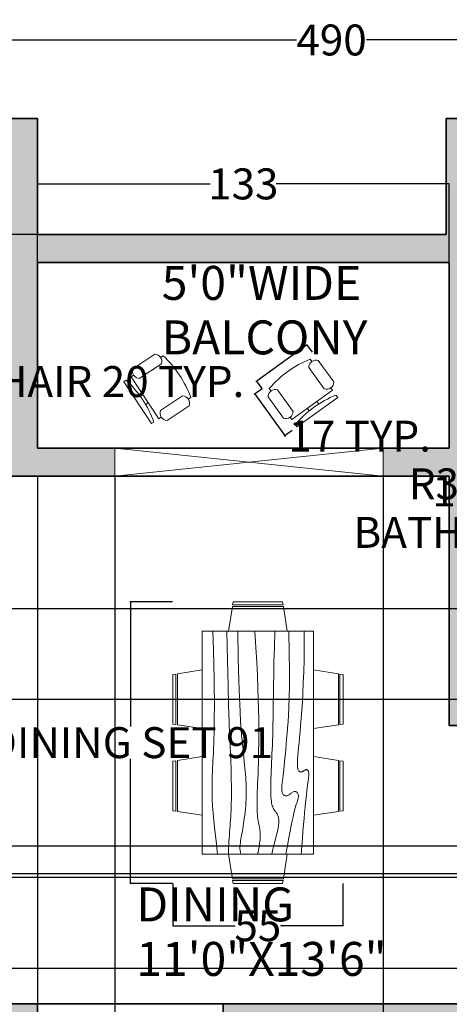
# Model space of a CAD drawing. Units: inches. Extents: x 143 to 746, y -392 to 145.
# Tile 3 of 6: x 334 to 473, y -173 to 145. Entities that reach past the tile are written whole.
import ezdxf

# ---------------------------------------------------------------- set-up
doc = ezdxf.new("R2010")
doc.units = ezdxf.units.IN
doc.header["$MEASUREMENT"] = 0
doc.linetypes.add('ACAD_ISO02W100', pattern=[15, 12, -3])
for name, color, linetype, lineweight in [('A-ANNO-DIMS', 2, 'Continuous', 18), ('A-AREA-IDEN', 7, 'Continuous', 20), ('A-DOOR', 3, 'Continuous', 18), ('A-FURN', 8, 'Continuous', 18), ('A-WALL', 7, 'Continuous', 35), ('A-WALL-OVHD', 7, 'ACAD_ISO02W100', 18)]:
    doc.layers.add(name, color=color, linetype=linetype, lineweight=lineweight)
doc.layers.add('A-WALL-PATT', color=252, linetype='Continuous', lineweight=13, true_color=0x939598)
doc.styles.get("Standard").update_dxf_attribs({"font": 'arial.ttf'})
doc.dimstyles.get("Standard").update_dxf_attribs({"dimtxt": 10, "dimasz": 0.18, "dimexe": 0.18, "dimexo": 0.0625, "dimgap": 0.09, "dimtad": 0, "dimtih": 1, "dimtoh": 1, "dimdec": 0, "dimzin": 0, "dimdsep": 46, "dimlunit": 3, "dimtxsty": 'Standard', "dimcen": 0.09, "dimadec": 0, "dimazin": 0, "dimtfac": 1, "dimtdec": 0, "dimtofl": 0, "dimtmove": 0, "dimatfit": 3, "dimfxl": 1, "dimtolj": 1, "dimtzin": 0, "dimarcsym": 0})

# ---------------------------------------------------------------- blocks, each defined once
blk = doc.blocks.new('Dining Set - 36 x 72 in.')
for p, q in [((-22.2343, 26.00059), (-23.4847, 17.99762)), ((-22.2304, 26), (-5.7608, 26)), ((-22, 27.5), (-22.1562, 26.50042)), ((-5.8416, 26.5), (-22.1534, 26.5)), ((-22, 27.5), (-6, 27.5)), ((-5.8437, 26.49966), (-6, 27.5)), ((-4.5152, 17.99762), (-5.7655, 25.99926)), ((5.7657, 26.00059), (4.5153, 17.99762)), ((5.7696, 26), (22.2392, 26)), ((6, 27.5), (5.8438, 26.50042)), ((22.1584, 26.5), (5.8466, 26.5)), ((6, 27.5), (22, 27.5)), ((22.1563, 26.49966), (22, 27.5)), ((23.4848, 17.99762), (22.2345, 25.99926)), ((36, 18), (-36, 18)), ((-36, 18), (-36, -18)), ((36, -18), (36, 18)), ((-45.5, 8), (-44.5004, 8.15617)), ((-45.5, 8), (-45.5, -8)), ((-44.5, -8.15843), (-44.5, 8.15338)), ((-44.0006, 8.23428), (-35.9976, 9.48474)), ((-44, 8.23041), (-44, -8.23915)), ((44.0006, 8.23428), (35.9976, 9.48474)), ((44, 8.23041), (44, -8.23915)), ((44.5, -8.15843), (44.5, 8.15338)), ((45.5, 8), (44.5005, 8.15617)), ((45.5, 8), (45.5, -8)), ((-44.4997, -8.15631), (-45.5, -8)), ((-35.9976, -9.48476), (-43.9993, -8.2345)), ((35.9976, -9.48476), (43.9993, -8.2345)), ((44.4997, -8.15631), (45.5, -8)), ((-36, -18), (36, -18)), ((-22.2343, -26.0006), (-23.4847, -17.99762)), ((-4.5152, -17.99762), (-5.7655, -25.99928)), ((5.7657, -26.0006), (4.5153, -17.99762)), ((23.4848, -17.99762), (22.2345, -25.99928)), ((-22.2304, -26), (-5.7608, -26)), ((-22, -27.5), (-22.1562, -26.50044)), ((-5.8416, -26.5), (-22.1534, -26.5)), ((-22, -27.5), (-6, -27.5)), ((-5.8437, -26.49967), (-6, -27.5)), ((5.7696, -26), (22.2392, -26)), ((6, -27.5), (5.8438, -26.50044)), ((22.1584, -26.5), (5.8466, -26.5)), ((6, -27.5), (22, -27.5)), ((22.1563, -26.49967), (22, -27.5))]:
    blk.add_line(p, q)
for points in [[(-36, 15), (-31.1772, 14.97754), (-26.8079, 14.91406), (-22.8538, 14.81543), (-19.276, 14.6875), (-16.0362, 14.53613), (-13.0957, 14.36718), (-10.4159, 14.18652), (-7.9583, 14), (-5.6904, 13.81315), (-3.6035, 13.63021), (-1.6954, 13.45508), (0.0365, 13.29166), (1.5945, 13.14388), (2.9811, 13.01562), (4.1988, 12.9108), (5.25, 12.83333), (6.1393, 12.78613), (6.8802, 12.76823), (7.4883, 12.77767), (7.9792, 12.8125), (8.3685, 12.87077), (8.6719, 12.95052), (8.9049, 13.0498), (9.0833, 13.16666), (9.2205, 13.29899), (9.3216, 13.44401), (9.3895, 13.59879), (9.4271, 13.76041), (9.4373, 13.92594), (9.4232, 14.09245), (9.3875, 14.257), (9.3333, 14.41666), (9.2638, 14.56917), (9.1836, 14.71484), (9.0975, 14.85465), (9.0104, 14.98958), (8.9272, 15.1206), (8.8529, 15.2487), (8.7922, 15.37483), (8.75, 15.5), (8.7305, 15.62467), (8.7344, 15.74739), (8.7617, 15.86621), (8.8125, 15.97916), (8.8867, 16.08431), (8.9844, 16.17968), (9.1055, 16.26334), (9.25, 16.33333), (9.4189, 16.38802), (9.6172, 16.42708), (9.8506, 16.45052), (10.125, 16.45833), (10.4463, 16.45052), (10.8203, 16.42708), (11.2529, 16.38802), (11.75, 16.33333), (12.3184, 16.26318), (12.9694, 16.17838), (13.7151, 16.07991), (14.5677, 15.96875), (15.5395, 15.84586), (16.6426, 15.71224), (17.8893, 15.56884), (19.2917, 15.41666), (20.859, 15.25667), (22.5879, 15.08984), (24.4721, 14.91715), (26.5052, 14.73958), (28.6809, 14.5581), (30.9929, 14.3737), (33.4347, 14.18733), (36, 14)], [(-36, 10), (-28.9766, 10.14274), (-23.1725, 10.20442), (-18.4241, 10.19775), (-14.5677, 10.13541), (-11.4399, 10.03011), (-8.877, 9.89453), (-6.7154, 9.74137), (-4.7917, 9.58333), (-2.9698, 9.43082), (-1.2246, 9.28515), (0.4415, 9.14534), (2.026, 9.01041), (3.5266, 8.87939), (4.9408, 8.7513), (6.266, 8.62516), (7.5, 8.5), (8.6411, 8.37549), (9.6914, 8.2539), (10.6538, 8.13818), (11.5312, 8.03125), (12.3267, 7.93603), (13.043, 7.85547), (13.6831, 7.79248), (14.25, 7.75), (14.7471, 7.7303), (15.1797, 7.73307), (15.5537, 7.75732), (15.875, 7.80208), (16.1494, 7.86637), (16.3828, 7.94922), (16.5811, 8.04964), (16.75, 8.16666), (16.8944, 8.29915), (17.0143, 8.44531), (17.1089, 8.60319), (17.1771, 8.77083), (17.218, 8.94629), (17.2305, 9.1276), (17.2137, 9.31282), (17.1667, 9.5), (17.0895, 9.6875), (16.987, 9.875), (16.8649, 10.0625), (16.7292, 10.25), (16.5856, 10.4375), (16.4401, 10.625), (16.2985, 10.8125), (16.1667, 11), (16.05, 11.18733), (15.9518, 11.3737), (15.8752, 11.5581), (15.8229, 11.73958), (15.798, 11.91715), (15.8034, 12.08984), (15.842, 12.25667), (15.9167, 12.41666), (16.0295, 12.56836), (16.1784, 12.70833), (16.3605, 12.83268), (16.5729, 12.9375), (16.8127, 13.01888), (17.0768, 13.07291), (17.3625, 13.0957), (17.6667, 13.08333), (17.9894, 13.03312), (18.3418, 12.94726), (18.7382, 12.82918), (19.1927, 12.68229), (19.7195, 12.51001), (20.3327, 12.31575), (21.0465, 12.10294), (21.875, 11.875), (22.8357, 11.63354), (23.959, 11.37304), (25.2786, 11.08618), (26.8282, 10.76562), (28.6414, 10.40405), (30.752, 9.99414), (33.1936, 9.52856), (36, 9)], [(-36, 5.5), (-30.7157, 5.3348), (-26.069, 5.20963), (-21.9946, 5.11767), (-18.4271, 5.05208), (-15.3009, 5.00602), (-12.5508, 4.97265), (-10.1112, 4.94515), (-7.9167, 4.91666), (-5.909, 4.88167), (-4.0586, 4.83984), (-2.3429, 4.79215), (-0.7396, 4.73958), (0.7739, 4.6831), (2.22, 4.6237), (3.6213, 4.56233), (5, 4.5), (6.373, 4.43782), (7.7344, 4.3776), (9.0723, 4.32129), (10.375, 4.27083), (11.6309, 4.22819), (12.8281, 4.19531), (13.9551, 4.17415), (15, 4.16666), (15.954, 4.17448), (16.819, 4.19791), (17.6001, 4.23698), (18.3021, 4.29166), (18.9299, 4.36198), (19.4883, 4.44791), (19.9823, 4.54948), (20.4167, 4.66666), (20.7969, 4.79899), (21.1302, 4.94401), (21.4245, 5.09879), (21.6875, 5.26041), (21.9271, 5.42594), (22.1511, 5.59245), (22.3672, 5.757), (22.5834, 5.91666), (22.8065, 6.06868), (23.0404, 6.21093), (23.2879, 6.34147), (23.5521, 6.45833), (23.8358, 6.55957), (24.142, 6.64323), (24.4735, 6.70735), (24.8334, 6.75), (25.2235, 6.76969), (25.642, 6.76692), (26.0858, 6.74267), (26.5521, 6.69791), (27.0379, 6.63362), (27.5404, 6.55078), (28.0565, 6.45036), (28.5834, 6.33333), (29.1242, 6.19987), (29.7071, 6.04687), (30.3661, 5.87044), (31.1354, 5.66666), (32.0493, 5.43164), (33.142, 5.16146), (34.4475, 4.85221), (36, 4.5)], [(-36, -1), (-30.7915, -0.6591), (-26.0195, -0.38216), (-21.6519, -0.16284), (-17.6563, 0.00521), (-14.0005, 0.12833), (-10.6523, 0.21289), (-7.5796, 0.26522), (-4.75, 0.29166), (-2.134, 0.29793), (0.2878, 0.28711), (2.5317, 0.26163), (4.6146, 0.22396), (6.5529, 0.17651), (8.3633, 0.12174), (10.0623, 0.06209), (11.6667, 0), (13.1899, -0.06201), (14.6341, -0.1211), (15.9982, -0.17432), (17.2813, -0.21875), (18.4823, -0.25147), (19.6003, -0.26953), (20.6343, -0.27002), (21.5834, -0.25), (22.4481, -0.20768), (23.2357, -0.14584), (23.9549, -0.06836), (24.6146, 0.02083), (25.2235, 0.11784), (25.7904, 0.21875), (26.3241, 0.31966), (26.8334, 0.41666), (27.3265, 0.50618), (27.8099, 0.58593), (28.2894, 0.65397), (28.7709, 0.70833), (29.2601, 0.74707), (29.763, 0.76823), (30.2855, 0.76985), (30.8334, 0.75), (31.4088, 0.70784), (31.9994, 0.64713), (32.589, 0.57275), (33.1615, 0.48958), (33.7008, 0.4025), (34.1908, 0.3164), (34.6153, 0.23616), (34.9584, 0.16666), (35.2099, 0.11165), (35.3848, 0.07031), (35.504, 0.04069), (35.5886, 0.02083), (35.6594, 0.00879), (35.7377, 0.0026), (35.8442, 0.00032), (36, 0)], [(-36, -6.5), (-27.1843, -6.31267), (-20.084, -6.1263), (-14.469, -5.9419), (-10.1094, -5.76042), (-6.7752, -5.58285), (-4.2363, -5.41016), (-2.2629, -5.24333), (-0.625, -5.08334), (0.8708, -4.93099), (2.2715, -4.78646), (3.5872, -4.64974), (4.8281, -4.52084), (6.0046, -4.39974), (7.127, -4.28646), (8.2053, -4.18099), (9.25, -4.08334), (10.2705, -3.99382), (11.2734, -3.91407), (12.2647, -3.84603), (13.25, -3.79167), (14.2354, -3.75293), (15.2266, -3.73177), (16.2295, -3.73015), (17.25, -3.75), (18.2912, -3.79248), (19.3451, -3.85547), (20.4009, -3.93604), (21.4479, -4.03125), (22.4754, -4.13819), (23.4727, -4.25391), (24.4289, -4.37549), (25.3334, -4.5), (26.1785, -4.62492), (26.9694, -4.74935), (27.7145, -4.87281), (28.4219, -4.99479), (29.1, -5.11483), (29.7572, -5.23242), (30.4016, -5.34709), (31.0417, -5.45834), (31.6837, -5.56437), (32.3262, -5.65821), (32.9658, -5.73153), (33.599, -5.77604), (34.2224, -5.78345), (34.8327, -5.74545), (35.4264, -5.65373), (36, -5.5)], [(-36, -10), (-26.4022, -9.81299), (-18.4675, -9.62891), (-11.9839, -9.45069), (-6.7396, -9.28125), (-2.5226, -9.12354), (0.8789, -8.98047), (3.6769, -8.85498), (6.0833, -8.75), (8.2767, -8.66765), (10.3021, -8.60677), (12.1712, -8.56543), (13.8958, -8.54167), (15.4876, -8.53353), (16.9583, -8.53907), (18.3197, -8.55632), (19.5834, -8.58334), (20.7616, -8.61841), (21.8685, -8.66081), (22.9188, -8.71004), (23.9271, -8.76563), (24.9081, -8.82707), (25.8763, -8.89388), (26.8465, -8.96558), (27.8334, -9.04167), (28.8474, -9.12118), (29.8828, -9.20117), (30.93, -9.27824), (31.9792, -9.34896), (33.0205, -9.40991), (34.0443, -9.45768), (35.0407, -9.48885), (36, -9.5)], [(-36, -14.5), (-30.0881, -14.33513), (-25.0332, -14.21224), (-20.7312, -14.12647), (-17.0781, -14.07292), (-13.97, -14.04671), (-11.3027, -14.04297), (-8.9724, -14.05681), (-6.875, -14.08334), (-4.9224, -14.11833), (-3.0905, -14.16016), (-1.3709, -14.20785), (0.2448, -14.26042), (1.7647, -14.3169), (3.1973, -14.3763), (4.5507, -14.43767), (5.8333, -14.5), (7.0554, -14.5621), (8.235, -14.62175), (9.3922, -14.67652), (10.5469, -14.72396), (11.7192, -14.76164), (12.929, -14.78711), (14.1965, -14.79794), (15.5417, -14.79167), (16.9933, -14.76424), (18.6152, -14.70508), (20.4804, -14.60197), (22.6615, -14.44271), (25.2312, -14.21509), (28.2624, -13.9069), (31.8277, -13.50594), (36, -13)]]:
    blk.add_lwpolyline(points)
blk = doc.blocks.new('Chair - Desk')
for p, q in [((-8.5, 0), (-8.5, -1)), ((-8.5, 0), (8.5, 0)), ((8.5, 0), (8.5, -1)), ((-8.5, -3), (-8.5, -4)), ((-8.5, -3), (8.5, -3)), ((-2, -3), (-2, -1.9355)), ((2, -1.9576), (2, -3)), ((8.5, -3), (8.5, -4)), ((-10.5, -5), (-10.5, -14)), ((-6.5, -14), (-6.5, -5)), ((6.5, -5), (6.5, -14)), ((10.5, -14), (10.5, -5)), ((-8.5, -15), (-8.5, -16)), ((8.5, -15), (8.5, -16))]:
    blk.add_line(p, q)
for centre, radius, start, end in [((0, 34.625), 36.625, 256.5803, 283.4197), ((-8.5, -6.5), 2.5, 36.8699, 143.1301), ((8.5, -6.5), 2.5, 36.8699, 143.1301), ((-8.5, -12.5), 2.5, 216.8699, 323.1301), ((0, 19.625), 36.625, 256.5803, 283.4197), ((8.5, -12.5), 2.5, 216.8699, 323.1301)]:
    blk.add_arc(centre, radius, start, end)
blk = doc.blocks.new('*D16')
at = {"layer": 'A-ANNO-DIMS', "color": 0, "lineweight": -2, "transparency": 16777216}
for p, q in [((493.94, -9.97), (497.14, -9.97)), ((496.96, -10.15), (496.96, -15.06)), ((496.96, -30.36), (496.96, -25.45)), ((493.94, -30.54), (497.14, -30.54))]:
    blk.add_line(p, q, dxfattribs=at)
at = {"layer": 'A-ANNO-DIMS', "color": 0, "transparency": 16777216}
for points in [[(496.93, -10.15), (496.99, -10.15), (496.96, -9.97)], [(496.93, -30.36), (496.99, -30.36), (496.96, -30.54)]]:
    blk.add_solid(points, dxfattribs=at)
at = {"layer": 'Defpoints', "color": 0, "transparency": 16777216}
for p in [(493.88, -9.97), (496.96, -9.97), (493.88, -30.54)]:
    blk.add_point(p, dxfattribs=at)
at = {"layer": 'A-ANNO-DIMS', "color": 0, "transparency": 16777216, "insert": (496.96, -20.25), "char_height": 10, "attachment_point": 5}
blk.add_mtext('\\A1;BATH FIXTURE 21', dxfattribs=at)
blk = doc.blocks.new('*D17')
at = {"layer": 'A-ANNO-DIMS', "color": 0, "lineweight": -2, "transparency": 16777216}
for p, q in [((481.54, -6.88), (481.36, -6.88)), ((481.54, -9.91), (481.54, -6.7)), ((493.7, -6.88), (481.72, -6.88)), ((493.88, -9.91), (493.88, -6.7))]:
    blk.add_line(p, q, dxfattribs=at)
at = {"layer": 'A-ANNO-DIMS', "color": 0, "transparency": 16777216}
for points in [[(481.72, -6.85), (481.72, -6.91), (481.54, -6.88)], [(493.7, -6.85), (493.7, -6.91), (493.88, -6.88)]]:
    blk.add_solid(points, dxfattribs=at)
at = {"layer": 'Defpoints', "color": 0, "transparency": 16777216}
for p in [(481.54, -6.88), (481.54, -9.97), (493.88, -9.97)]:
    blk.add_point(p, dxfattribs=at)
at = {"layer": 'A-ANNO-DIMS', "color": 0, "transparency": 16777216, "insert": (474.63, -6.88), "char_height": 10, "attachment_point": 5}
blk.add_mtext('\\A1;12', dxfattribs=at)
blk = doc.blocks.new('*D18')
at = {"layer": 'A-ANNO-DIMS', "color": 0, "lineweight": -2, "transparency": 16777216}
for p, q in [((426.49, 40.22), (410.54, 28.71)), ((428.36, 37.94), (426.53, 40.48)), ((412.12, 26.22), (410.29, 28.75)), ((410.25, 28.5), (410.07, 28.5)), ((410.4, 28.6), (410.25, 28.5))]:
    blk.add_line(p, q, dxfattribs=at)
at = {"layer": 'A-ANNO-DIMS', "color": 0, "transparency": 16777216}
for points in [[(426.47, 40.25), (426.51, 40.2), (426.64, 40.33)], [(410.53, 28.73), (410.56, 28.68), (410.4, 28.6)]]:
    blk.add_solid(points, dxfattribs=at)
at = {"layer": 'Defpoints', "color": 0, "transparency": 16777216}
for p in [(428.4, 37.89), (410.4, 28.6), (412.16, 26.17)]:
    blk.add_point(p, dxfattribs=at)
at = {"layer": 'A-ANNO-DIMS', "color": 0, "transparency": 16777216, "insert": (362.03, 28.5), "char_height": 10, "attachment_point": 5}
blk.add_mtext('\\A1;CHAIR 20 TYP.', dxfattribs=at)
blk = doc.blocks.new('*D19')
at = {"layer": 'A-ANNO-DIMS', "color": 0, "lineweight": -2, "transparency": 16777216}
for p, q in [((412.11, 26.13), (409.58, 24.3)), ((409.83, 24.26), (419.3, 11.15)), ((421.79, 12.73), (419.25, 10.9)), ((419.4, 11.01), (419.51, 10.86)), ((419.51, 10.86), (419.69, 10.86))]:
    blk.add_line(p, q, dxfattribs=at)
at = {"layer": 'A-ANNO-DIMS', "color": 0, "transparency": 16777216}
for points in [[(409.85, 24.28), (409.8, 24.25), (409.72, 24.41)], [(419.32, 11.17), (419.27, 11.13), (419.4, 11.01)]]:
    blk.add_solid(points, dxfattribs=at)
at = {"layer": 'Defpoints', "color": 0, "transparency": 16777216}
for p in [(412.16, 26.17), (421.84, 12.76), (419.4, 11.01)]:
    blk.add_point(p, dxfattribs=at)
at = {"layer": 'A-ANNO-DIMS', "color": 0, "transparency": 16777216, "insert": (443.64, 10.86), "char_height": 10, "attachment_point": 5}
blk.add_mtext('\\A1;17 TYP.', dxfattribs=at)
blk = doc.blocks.new('*D32')
at = {"layer": 'A-ANNO-DIMS', "color": 0, "lineweight": -2, "transparency": 16777216}
for p, q in [((383.18, -42.7), (369.41, -42.7)), ((369.59, -42.88), (369.59, -82.94)), ((369.59, -133.52), (369.59, -93.46)), ((383.18, -133.7), (369.41, -133.7))]:
    blk.add_line(p, q, dxfattribs=at)
at = {"layer": 'A-ANNO-DIMS', "color": 0, "transparency": 16777216}
for points in [[(369.56, -42.88), (369.62, -42.88), (369.59, -42.7)], [(369.56, -133.52), (369.62, -133.52), (369.59, -133.7)]]:
    blk.add_solid(points, dxfattribs=at)
at = {"layer": 'Defpoints', "color": 0, "transparency": 16777216}
for p in [(383.24, -42.7), (369.59, -133.7), (383.24, -133.7)]:
    blk.add_point(p, dxfattribs=at)
at = {"layer": 'A-ANNO-DIMS', "color": 0, "transparency": 16777216, "insert": (369.59, -88.2), "char_height": 10, "attachment_point": 5}
blk.add_mtext('\\A1;DINING SET 91', dxfattribs=at)
blk = doc.blocks.new('*D33')
at = {"layer": 'A-ANNO-DIMS', "color": 0, "lineweight": -2, "transparency": 16777216}
for p, q in [((383.24, -133.76), (383.24, -147.53)), ((438.24, -133.76), (438.24, -147.53)), ((383.42, -147.35), (403.45, -147.35)), ((438.06, -147.35), (418.03, -147.35))]:
    blk.add_line(p, q, dxfattribs=at)
at = {"layer": 'A-ANNO-DIMS', "color": 0, "transparency": 16777216}
for points in [[(383.42, -147.32), (383.42, -147.38), (383.24, -147.35)], [(438.06, -147.32), (438.06, -147.38), (438.24, -147.35)]]:
    blk.add_solid(points, dxfattribs=at)
at = {"layer": 'Defpoints', "color": 0, "transparency": 16777216}
for p in [(383.24, -133.7), (438.24, -133.7), (438.24, -147.35)]:
    blk.add_point(p, dxfattribs=at)
at = {"layer": 'A-ANNO-DIMS', "color": 0, "transparency": 16777216, "insert": (410.74, -147.35), "char_height": 10, "attachment_point": 5}
blk.add_mtext('\\A1;55', dxfattribs=at)
blk = doc.blocks.new('*D43')
at = {"layer": 'A-ANNO-DIMS', "color": 0, "lineweight": -2, "transparency": 16777216}
for p, q in [((189.54, 28.45), (189.54, 139.06)), ((189.72, 138.88), (423.22, 138.88)), ((679.36, 138.88), (445.86, 138.88)), ((679.54, 31.45), (679.54, 139.06))]:
    blk.add_line(p, q, dxfattribs=at)
at = {"layer": 'A-ANNO-DIMS', "color": 0, "transparency": 16777216}
for points in [[(189.72, 138.91), (189.72, 138.85), (189.54, 138.88)], [(679.36, 138.91), (679.36, 138.85), (679.54, 138.88)]]:
    blk.add_solid(points, dxfattribs=at)
at = {"layer": 'Defpoints', "color": 0, "transparency": 16777216}
for p in [(679.54, 138.88), (679.54, 31.39), (189.54, 28.39)]:
    blk.add_point(p, dxfattribs=at)
at = {"layer": 'A-ANNO-DIMS', "color": 0, "transparency": 16777216, "insert": (434.54, 138.88), "char_height": 10, "attachment_point": 5}
blk.add_mtext('\\A1;490', dxfattribs=at)
blk = doc.blocks.new('*D44')
at = {"layer": 'A-ANNO-DIMS', "color": 0, "lineweight": -2, "transparency": 16777216}
for p, q in [((189.6, -131.67), (718.91, -131.67)), ((718.73, -131.85), (718.73, -146.94)), ((718.73, -172.43), (718.73, -157.34)), ((198.6, -172.61), (718.91, -172.61))]:
    blk.add_line(p, q, dxfattribs=at)
at = {"layer": 'A-ANNO-DIMS', "color": 0, "transparency": 16777216}
for points in [[(718.7, -131.85), (718.76, -131.85), (718.73, -131.67)], [(718.7, -172.43), (718.76, -172.43), (718.73, -172.61)]]:
    blk.add_solid(points, dxfattribs=at)
at = {"layer": 'Defpoints', "color": 0, "transparency": 16777216}
for p in [(189.54, -131.67), (718.73, -131.67), (198.54, -172.61)]:
    blk.add_point(p, dxfattribs=at)
at = {"layer": 'A-ANNO-DIMS', "color": 0, "transparency": 16777216, "insert": (718.73, -152.14), "char_height": 10, "attachment_point": 5}
blk.add_mtext('\\A1;40.935', dxfattribs=at)
blk = doc.blocks.new('*D49')
at = {"layer": 'A-ANNO-DIMS', "color": 0, "lineweight": -2, "transparency": 16777216}
for p, q in [((339.54, 67.03), (339.54, 92.55)), ((339.72, 92.37), (395.37, 92.37)), ((472.36, 92.37), (416.7, 92.37)), ((472.54, 67.03), (472.54, 92.55))]:
    blk.add_line(p, q, dxfattribs=at)
at = {"layer": 'A-ANNO-DIMS', "color": 0, "transparency": 16777216}
for points in [[(339.72, 92.4), (339.72, 92.34), (339.54, 92.37)], [(472.36, 92.4), (472.36, 92.34), (472.54, 92.37)]]:
    blk.add_solid(points, dxfattribs=at)
at = {"layer": 'Defpoints', "color": 0, "transparency": 16777216}
for p in [(472.54, 92.37), (339.54, 66.97), (472.54, 66.97)]:
    blk.add_point(p, dxfattribs=at)
at = {"layer": 'A-ANNO-DIMS', "color": 0, "transparency": 16777216, "insert": (406.04, 92.37), "char_height": 10, "attachment_point": 5}
blk.add_mtext('\\A1;133', dxfattribs=at)
blk = doc.blocks.new('*D50')
at = {"layer": 'A-ANNO-DIMS', "color": 0, "lineweight": -2, "transparency": 16777216}
for p, q in [((339.48, 113.48), (313.96, 113.48)), ((314.14, 113.3), (314.14, 99.92)), ((314.14, 76.15), (314.14, 89.52)), ((339.48, 75.97), (313.96, 75.97))]:
    blk.add_line(p, q, dxfattribs=at)
at = {"layer": 'A-ANNO-DIMS', "color": 0, "transparency": 16777216}
for points in [[(314.11, 113.3), (314.17, 113.3), (314.14, 113.48)], [(314.11, 76.15), (314.17, 76.15), (314.14, 75.97)]]:
    blk.add_solid(points, dxfattribs=at)
at = {"layer": 'Defpoints', "color": 0, "transparency": 16777216}
for p in [(314.14, 113.48), (339.54, 113.48), (339.54, 75.97)]:
    blk.add_point(p, dxfattribs=at)
at = {"layer": 'A-ANNO-DIMS', "color": 0, "transparency": 16777216, "insert": (314.14, 94.72), "char_height": 10, "attachment_point": 5}
blk.add_mtext('\\A1;37.51', dxfattribs=at)
blk = doc.blocks.new('*D51')
at = {"layer": 'A-ANNO-DIMS', "color": 0, "lineweight": -2, "transparency": 16777216}
for p, q in [((339.54, -2.09), (339.54, -385.98)), ((364.51, -2.09), (364.51, -385.98)), ((339.72, -385.8), (364.33, -385.8)), ((364.51, -385.8), (364.69, -385.8))]:
    blk.add_line(p, q, dxfattribs=at)
at = {"layer": 'A-ANNO-DIMS', "color": 0, "transparency": 16777216}
for points in [[(339.72, -385.77), (339.72, -385.83), (339.54, -385.8)], [(364.33, -385.77), (364.33, -385.83), (364.51, -385.8)]]:
    blk.add_solid(points, dxfattribs=at)
at = {"layer": 'Defpoints', "color": 0, "transparency": 16777216}
for p in [(339.54, -2.03), (364.51, -2.03), (364.51, -385.8)]:
    blk.add_point(p, dxfattribs=at)
at = {"layer": 'A-ANNO-DIMS', "color": 0, "transparency": 16777216, "insert": (381.74, -385.8), "char_height": 10, "attachment_point": 5}
blk.add_mtext('\\A1;24.97', dxfattribs=at)
blk = doc.blocks.new('*D52')
at = {"layer": 'A-ANNO-DIMS', "color": 0, "lineweight": -2, "transparency": 16777216}
for p, q in [((364.51, -2.09), (364.51, -385.98)), ((451.23, -2.09), (451.23, -385.98)), ((364.69, -385.8), (390.95, -385.8)), ((451.05, -385.8), (424.79, -385.8))]:
    blk.add_line(p, q, dxfattribs=at)
at = {"layer": 'A-ANNO-DIMS', "color": 0, "transparency": 16777216}
for points in [[(364.69, -385.77), (364.69, -385.83), (364.51, -385.8)], [(451.05, -385.77), (451.05, -385.83), (451.23, -385.8)]]:
    blk.add_solid(points, dxfattribs=at)
at = {"layer": 'Defpoints', "color": 0, "transparency": 16777216}
for p in [(364.51, -2.03), (451.23, -2.03), (451.23, -385.8)]:
    blk.add_point(p, dxfattribs=at)
at = {"layer": 'A-ANNO-DIMS', "color": 0, "transparency": 16777216, "insert": (407.87, -385.8), "char_height": 10, "attachment_point": 5}
blk.add_mtext('\\A1;86.72', dxfattribs=at)
blk = doc.blocks.new('*D67')
at = {"layer": 'A-ANNO-DIMS', "color": 0, "lineweight": -2, "transparency": 16777216}
for p, q in [((528.48, -121.61), (163.96, -121.61)), ((164.14, -121.79), (164.14, -130.43)), ((528.48, -130.61), (163.96, -130.61)), ((164.14, -130.79), (163.96, -130.79)), ((164.14, -130.61), (164.14, -130.79))]:
    blk.add_line(p, q, dxfattribs=at)
at = {"layer": 'A-ANNO-DIMS', "color": 0, "transparency": 16777216}
for points in [[(164.11, -121.79), (164.17, -121.79), (164.14, -121.61)], [(164.11, -130.43), (164.17, -130.43), (164.14, -130.61)]]:
    blk.add_solid(points, dxfattribs=at)
at = {"layer": 'Defpoints', "color": 0, "transparency": 16777216}
for p in [(528.54, -121.61), (164.14, -130.61), (528.54, -130.61)]:
    blk.add_point(p, dxfattribs=at)
at = {"layer": 'A-ANNO-DIMS', "color": 0, "transparency": 16777216, "insert": (160.58, -130.79), "char_height": 10, "attachment_point": 5}
blk.add_mtext('\\A1;9', dxfattribs=at)
blk = doc.blocks.new('*D69')
at = {"layer": 'A-ANNO-DIMS', "color": 0, "lineweight": -2, "transparency": 16777216}
for p, q in [((284.99, -44.86), (718.91, -44.86)), ((718.73, -45.04), (718.73, -54.32)), ((718.73, -73.99), (718.73, -64.72)), ((284.99, -74.17), (718.91, -74.17))]:
    blk.add_line(p, q, dxfattribs=at)
at = {"layer": 'A-ANNO-DIMS', "color": 0, "transparency": 16777216}
for points in [[(718.7, -45.04), (718.76, -45.04), (718.73, -44.86)], [(718.7, -73.99), (718.76, -73.99), (718.73, -74.17)]]:
    blk.add_solid(points, dxfattribs=at)
at = {"layer": 'Defpoints', "color": 0, "transparency": 16777216}
for p in [(284.93, -44.86), (284.93, -74.17), (718.73, -74.17)]:
    blk.add_point(p, dxfattribs=at)
at = {"layer": 'A-ANNO-DIMS', "color": 0, "transparency": 16777216, "insert": (718.73, -59.52), "char_height": 10, "attachment_point": 5}
blk.add_mtext('\\A1;29.31', dxfattribs=at)
blk = doc.blocks.new('*D70')
at = {"layer": 'A-ANNO-DIMS', "color": 0, "lineweight": -2, "transparency": 16777216}
for p, q in [((645.96, -161.14), (163.96, -161.14)), ((164.14, -161.32), (164.14, -167.24)), ((164.14, -183.56), (164.14, -177.64)), ((645.96, -183.74), (163.96, -183.74))]:
    blk.add_line(p, q, dxfattribs=at)
at = {"layer": 'A-ANNO-DIMS', "color": 0, "transparency": 16777216}
for points in [[(164.11, -161.32), (164.17, -161.32), (164.14, -161.14)], [(164.11, -183.56), (164.17, -183.56), (164.14, -183.74)]]:
    blk.add_solid(points, dxfattribs=at)
at = {"layer": 'Defpoints', "color": 0, "transparency": 16777216}
for p in [(646.02, -161.14), (164.14, -183.74), (646.02, -183.74)]:
    blk.add_point(p, dxfattribs=at)
at = {"layer": 'A-ANNO-DIMS', "color": 0, "transparency": 16777216, "insert": (164.14, -172.44), "char_height": 10, "attachment_point": 5}
blk.add_mtext('\\A1;22.604', dxfattribs=at)
blk = doc.blocks.new('*D75')
at = {"layer": 'A-ANNO-DIMS', "color": 0, "lineweight": -2, "transparency": 16777216}
for p, q in [((528.48, -130.61), (163.96, -130.61)), ((164.14, -130.79), (164.14, -146.5)), ((164.14, -172.43), (164.14, -156.72)), ((528.48, -172.61), (163.96, -172.61))]:
    blk.add_line(p, q, dxfattribs=at)
at = {"layer": 'A-ANNO-DIMS', "color": 0, "transparency": 16777216}
for points in [[(164.11, -130.79), (164.17, -130.79), (164.14, -130.61)], [(164.11, -172.43), (164.17, -172.43), (164.14, -172.61)]]:
    blk.add_solid(points, dxfattribs=at)
at = {"layer": 'Defpoints', "color": 0, "transparency": 16777216}
for p in [(164.14, -130.61), (528.54, -130.61), (528.54, -172.61)]:
    blk.add_point(p, dxfattribs=at)
at = {"layer": 'A-ANNO-DIMS', "color": 0, "transparency": 16777216, "insert": (164.14, -151.61), "char_height": 10, "attachment_point": 5}
blk.add_mtext('\\A1;42', dxfattribs=at)
blk = doc.blocks.new('*D79')
at = {"layer": 'A-ANNO-DIMS', "color": 0, "lineweight": -2, "transparency": 16777216}
for p, q in [((510.28, -4.57), (510.46, -4.57)), ((510.46, -4.57), (522.99, -17.23)), ((544.13, -38.69), (544.31, -38.69)), ((544.22, -38.78), (544.22, -38.6))]:
    blk.add_line(p, q, dxfattribs=at)
at = {"layer": 'A-ANNO-DIMS', "color": 0, "transparency": 16777216}
blk.add_solid([(523.01, -17.21), (522.97, -17.25), (523.12, -17.36)], dxfattribs=at)
at = {"layer": 'Defpoints', "color": 0, "transparency": 16777216}
for p in [(523.12, -17.36), (544.22, -38.69)]:
    blk.add_point(p, dxfattribs=at)
at = {"layer": 'A-ANNO-DIMS', "color": 0, "transparency": 16777216, "insert": (484.64, -4.57), "char_height": 10, "attachment_point": 5}
blk.add_mtext('\\A1;R30.003', dxfattribs=at)

msp = doc.modelspace()

# ---------------------------------------------------------------- hatches: boundary and pattern name
at = {"layer": 'A-WALL-PATT'}
h = msp.add_hatch(color=256, dxfattribs=at)
h.dxf.hatch_style = 1
h.paths.add_polyline_path([(198.538, 19.3924), (257.4275, 19.3924), (257.4275, 28.3924), (189.538, 28.3924), (189.538, -95.6731, -0.06325422), (198.538, -96.8162)])
h.paths.add_polyline_path([(339.538, 66.969), (471.538, 66.969), (472.538, 66.969), (472.538, 31.3924), (472.538, 6.969), (451.2296, 6.969), (451.2296, -2.031), (472.538, -2.031), (472.538, -82.6076), (544.538, -82.6076), (544.538, -38.6894), (535.538, -38.6894), (535.538, -73.6076), (481.538, -73.6076), (481.538, 22.3924), (498.7149, 22.3924), (498.7149, 31.3924), (481.538, 31.3924), (481.538, 66.969), (481.538, 113.4779), (471.538, 113.4779), (471.538, 75.969), (339.538, 75.969), (339.538, 113.4779), (330.538, 113.4779), (330.538, 66.969), (330.538, 28.3924), (293.6446, 28.3924), (293.6446, 19.3924), (330.538, 19.3924), (330.538, 6.969), (330.538, -2.031), (364.5099, -2.031), (364.5099, 6.969), (339.538, 6.969)])
h.paths.add_polyline_path([(570.63, 31.3924), (544.538, 31.3924), (524.7988, 31.3924), (524.7988, 22.3924), (535.538, 22.3924), (535.538, -9.9696, -0.0761882), (544.538, -8.6878), (544.538, 22.3924), (570.63, 22.3924)])
h.paths.add_polyline_path([(679.538, 31.3924), (618.768, 31.3924), (618.768, 22.3924), (670.538, 22.3924), (670.538, -54.5218), (679.538, -54.5218)])
h.paths.add_polyline_path([(679.538, -90.0753), (670.538, -90.0753), (670.538, -121.6076), (537.538, -121.6076), (528.538, -121.6076), (528.538, -130.6076), (537.538, -130.6076), (670.538, -130.6076), (670.538, -150.8923), (679.538, -150.8923)])
h.paths.add_polyline_path([(679.538, -187.0502), (670.538, -187.0502), (670.538, -232.6076), (636.538, -232.6076, -0.07632083), (635.1562, -241.6076), (670.538, -241.6076), (670.538, -256.599), (679.538, -256.599)])
h.paths.add_polyline_path([(606.538, -232.6076), (537.538, -232.6076), (537.538, -241.6076), (597.538, -241.6076), (597.538, -337.6076), (590.545, -337.6076), (590.545, -346.6076), (679.538, -346.6076), (679.538, -316.1251), (670.538, -316.1251), (670.538, -337.6076), (606.538, -337.6076)])
h.paths.add_polyline_path([(537.538, -181.6076), (537.538, -172.6076), (528.538, -172.6076), (528.538, -209.005), (528.538, -269.6672, -0.07632083), (537.538, -271.0491)])
h.paths.add_polyline_path([(566.8252, -337.6076), (537.538, -337.6076), (537.538, -299.6672), (528.538, -299.6672), (528.538, -337.6076), (513.484, -337.6076), (513.484, -346.6076), (566.8252, -346.6076)])
h.paths.add_polyline_path([(477.1278, -337.6076), (408.538, -337.6076), (408.538, -229.6076), (408.538, -181.6076), (493.5793, -181.6076, -0.06316411), (492.538, -172.6076), (399.538, -172.6076), (399.538, -229.6076), (399.538, -337.6076), (388.659, -337.6076), (388.659, -346.6076), (477.1278, -346.6076)])
h.paths.add_polyline_path([(364.4504, -337.6076), (339.538, -337.6076), (339.538, -301.3371), (330.538, -301.3371), (330.538, -337.6076), (307.2736, -337.6076), (307.2736, -346.6076), (364.4504, -346.6076)])
h.paths.add_polyline_path([(339.538, -229.6076), (399.538, -229.6076), (399.538, -220.6076), (369.1898, -220.6076), (330.538, -220.6076), (330.538, -271.2389, -0.07612824), (339.538, -272.6672)])
h.paths.add_polyline_path([(271.3704, -337.6076), (198.538, -337.6076), (198.538, -181.6076), (339.538, -181.6076), (339.538, -172.6076), (198.538, -172.6076), (198.538, -131.6731), (189.538, -131.6731), (189.538, -346.6076), (271.3704, -346.6076)])

# ---------------------------------------------------------------- linework, layer by layer
at = {"layer": 'A-DOOR'}
for p, q in [((364.5099, 6.969), (364.5099, -2.031)), ((451.2296, 6.969), (364.5099, -2.031)), ((451.2296, -2.031), (364.5099, 6.969)), ((451.2296, 6.969), (451.2296, -2.031))]:
    msp.add_line(p, q, dxfattribs=at)
at = {"layer": 'A-WALL'}
for p, q in [((339.538, 113.4779), (330.538, 113.4779)), ((339.538, 75.969), (339.538, 113.4779)), ((471.538, 75.969), (471.538, 113.4779)), ((471.538, 113.4779), (481.538, 113.4779)), ((339.538, 75.969), (471.538, 75.969)), ((339.538, 6.969), (339.538, 66.969)), ((339.538, 66.969), (471.538, 66.969)), ((471.538, 66.969), (472.538, 66.969)), ((472.538, 66.969), (472.538, 31.3924)), ((472.538, 6.969), (472.538, 31.3924)), ((339.538, 6.969), (339.538, 19.3924)), ((472.538, 6.969), (339.538, 6.969)), ((472.538, -2.031), (330.538, -2.031)), ((472.538, -82.6076), (472.538, -2.031)), ((544.538, -82.6076), (472.538, -82.6076)), ((198.538, -172.6076), (339.538, -172.6076)), ((339.538, -181.6076), (339.538, -172.6076)), ((399.538, -172.6076), (399.538, -229.6076)), ((492.538, -172.6076), (399.538, -172.6076))]:
    msp.add_line(p, q, dxfattribs=at)
at = {"layer": 'A-WALL-OVHD'}
for q in [(339.538, -2.031), (399.538, -172.6076)]:
    msp.add_line((339.538, -172.6076), q, dxfattribs=at)

# ---------------------------------------------------------------- block references
at = {"layer": 'A-FURN', "xscale": 0.9538052522890815, "yscale": 0.9538052522890815, "zscale": 0.9538052522890815}
for p, rotation in [((371.9006, 21.6554), 123.5325031950965), ((429.9558, 18.6275), 215.8343509099021)]:
    msp.add_blockref('Chair - Desk', p, dxfattribs=dict(at, rotation=rotation))
at = {"layer": 'A-FURN', "rotation": 270}
msp.add_blockref('Dining Set - 36 x 72 in.', (410.7422, -88.1958), dxfattribs=at)

# ---------------------------------------------------------------- texts
at = {"layer": 'A-AREA-IDEN'}
for s, height, p in [('5\'0"WIDE', 10.95807, (379.7016, 54.9003)), ('BALCONY', 10.95807, (379.7016, 37.2972)), ('DINING', 10.95807, (371.481, -145.9593)), ('11\'0"X13\'6"', 10.958074, (371.481, -163.5624))]:
    msp.add_text(s, height=height, dxfattribs=at).set_placement(p)

# ---------------------------------------------------------------- dimensions: what is measured, and where the dimension line sits
at = {"layer": 'A-ANNO-DIMS'}
for base, p1, p2, override, picture, middle in [((679.538, 138.8779), (189.538, 28.3924), (679.538, 31.3924), {"dimdec": 0, "dimlfac": 1, "dimrnd": 0, "dimzin": 0, "dimdsep": 46, "dimlunit": 2}, '*D43', (434.538, 138.8779)), ((472.538, 92.369), (339.538, 66.969), (472.538, 66.969), {"dimdec": 0, "dimlfac": 1, "dimrnd": 0, "dimzin": 0, "dimdsep": 46, "dimlunit": 2}, '*D49', (406.038, 92.369)), ((364.5099, -385.7951), (339.538, -2.031), (364.5099, -2.031), {"dimdec": 2, "dimlfac": 1, "dimrnd": 0, "dimzin": 0, "dimdsep": 46, "dimlunit": 2}, '*D51', (381.7376, -385.7951)), ((451.2296, -385.7951), (364.5099, -2.031), (451.2296, -2.031), {"dimdec": 2, "dimlfac": 1, "dimrnd": 0, "dimzin": 0, "dimdsep": 46, "dimlunit": 2}, '*D52', (407.8698, -385.7951)), ((438.2422, -147.3458), (383.2422, -133.6958), (438.2422, -133.6958), {"dimdec": 0, "dimlfac": 1, "dimrnd": 0, "dimzin": 0, "dimdsep": 46, "dimlunit": 2}, '*D33', (410.7422, -147.3458))]:
    dim = msp.add_linear_dim(base=base, p1=p1, p2=p2, dimstyle='Standard', override=override, dxfattribs=at)
    dim.commit()
    dim.dimension.update_dxf_attribs({"geometry": picture, "text_midpoint": middle})
for base, p1, p2, angle, override, picture, middle in [((314.138, 113.4779), (339.538, 75.969), (339.538, 113.4779), 90, {"dimdec": 2, "dimlfac": 1, "dimrnd": 0, "dimzin": 0, "dimdsep": 46, "dimlunit": 2}, '*D50', (314.138, 94.7234)), ((481.538, -6.8845), (493.8785, -9.9696), (481.538, -9.9696), 180, {"dimdec": 0, "dimlfac": 1, "dimrnd": 0, "dimzin": 0, "dimdsep": 46, "dimlunit": 2}, '*D17', (474.6275, -6.8845)), ((718.7255, -74.1707), (284.9288, -44.8632), (284.9288, -74.1707), 90, {"dimdec": 2, "dimlfac": 1, "dimrnd": 0, "dimzin": 0, "dimdsep": 46, "dimlunit": 2}, '*D69', (718.7255, -59.5169)), ((164.138, -130.6076), (528.538, -121.6076), (528.538, -130.6076), 90, {"dimdec": 0, "dimlfac": 1, "dimrnd": 0, "dimzin": 0, "dimdsep": 46, "dimlunit": 2}, '*D67', (160.5802, -130.7876)), ((164.138, -130.6076), (528.538, -172.6076), (528.538, -130.6076), 90, {"dimdec": 0, "dimlfac": 1, "dimrnd": 0, "dimzin": 0, "dimdsep": 46, "dimlunit": 2}, '*D75', (164.138, -151.6076)), ((718.72548, -131.67308), (198.53803, -172.6076), (189.53803, -131.67308), 90, {"dimdec": 3, "dimlfac": 1, "dimrnd": 0, "dimzin": 0, "dimdsep": 46, "dimlunit": 2}, '*D44', (718.72548, -152.14034)), ((164.138, -183.7414), (646.0181, -161.1374), (646.0181, -183.7414), 90, {"dimdec": 3, "dimlfac": 1, "dimrnd": 0, "dimzin": 0, "dimdsep": 46, "dimlunit": 2}, '*D70', (164.138, -172.4394))]:
    dim = msp.add_linear_dim(base=base, p1=p1, p2=p2, angle=angle, dimstyle='Standard', override=override, dxfattribs=at)
    dim.commit()
    dim.dimension.update_dxf_attribs({"geometry": picture, "text_midpoint": middle})
for base, p1, p2, angle, text, picture, middle in [((410.3987, 28.6033), (428.3961, 37.8939), (412.1576, 26.1675), 215.834351, 'CHAIR <> TYP.', '*D18', (362.0291, 28.4979)), ((419.4008, 11.0054), (412.1576, 26.1675), (421.8365, 12.7643), 305.834351, '<> TYP.', '*D19', (443.6438, 10.8594)), ((496.9636, -9.9696), (493.8785, -30.5371), (493.8785, -9.9696), 90, 'BATH FIXTURE <>', '*D16', (496.9636, -20.2533)), ((369.5922, -133.6958), (383.2422, -42.6958), (383.2422, -133.6958), 270, 'DINING SET <>', '*D32', (369.5922, -88.1958))]:
    dim = msp.add_linear_dim(base=base, p1=p1, p2=p2, angle=angle, text=text, dimstyle='Standard', override={"dimdec": 0, "dimlfac": 1, "dimrnd": 0, "dimzin": 0, "dimdsep": 46, "dimlunit": 2}, dxfattribs=at)
    dim.commit()
    dim.dimension.update_dxf_attribs({"geometry": picture, "text_midpoint": middle})
dim = msp.add_radius_dim(center=(544.2196, -38.6894), mpoint=(523.1168, -17.3618), dimstyle='Standard', override={"dimdec": 3, "dimlfac": 1, "dimrnd": 0, "dimzin": 0, "dimdsep": 46, "dimlunit": 2}, dxfattribs=at)
dim.commit()
dim.dimension.update_dxf_attribs({"geometry": '*D79', "text_midpoint": (484.6428, -4.5652), "dimtype": 164})

doc.saveas('drawing.dxf')
